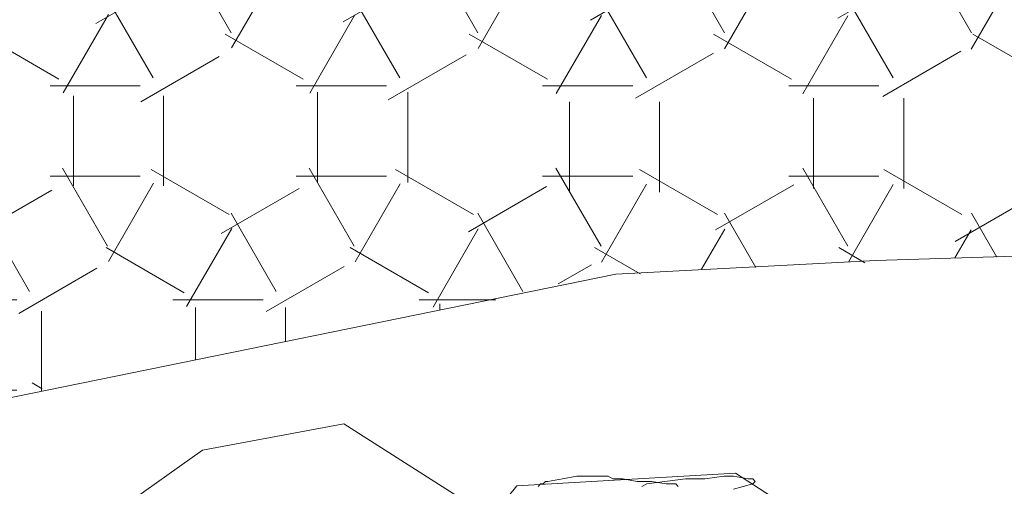
# Model space of a CAD drawing. Units: inches. Extents: x 1994 to 3075, y 3517 to 3950.
# Tile 42 of 58: x 1994.63804 to 1994.65094, y 3553.74931 to 3553.75542. Entities that reach past the tile are written whole.
import ezdxf

# ---------------------------------------------------------------- set-up
doc = ezdxf.new("R2010")
doc.units = ezdxf.units.IN
doc.layers.add('A-FURN-REFR', color=8, linetype='Continuous', lineweight=13)
doc.layers.add('A-FURN-REFR-PATT', color=8, linetype='Continuous', lineweight=13)

msp = doc.modelspace()

# ---------------------------------------------------------------- hatches: boundary and pattern name
at = {"layer": 'A-FURN-REFR-PATT'}
h = msp.add_hatch(dxfattribs=at)
h.set_pattern_fill('ESA_QT1', color=256, scale=0.001181, style=0, pattern_type=2)
h.set_pattern_definition([(0, (2000.7131367, 3549.95567), (0.0016133858, 0.0027944882), [0.0011811024, -0.0020457874]), (0, (2000.7131367, 3549.956851), (0.0016133858, 0.0027944882), [0.0011811024, -0.0020457874]), (60, (2000.7147507, 3549.9540566), (-0.0016134048, 0.0027944772), [0.0011811024, -0.0020457874]), (60, (2000.7137272, 3549.9546472), (-0.0016134048, 0.0027944772), [0.0011811024, -0.0020457874]), (120, (2000.7159311, 3549.9540566), (-0.0032267907, -1.1e-08), [0.0011811024, -0.0020457874]), (120, (2000.716954, 3549.9546472), (-0.0032267907, -1.1e-08), [0.0011811024, -0.0020457874]), (90, (2000.7131367, 3549.95567), (-0.00161338583, 0.0027944882), [0.0011811024, -0.0044079921]), (90, (2000.7143178, 3549.95567), (-0.00161338583, 0.0027944882), [0.0011811024, -0.0044079921]), (30, (2000.7159311, 3549.9540566), (0.00161340485, 0.0027944772), [0.0011811024, -0.0044079921]), (150, (2000.71475, 3549.9540566), (-0.00322679068, 1.1e-08), [0.0011811024, -0.0044079921]), (30, (2000.7153406, 3549.9550795), (0.00161340485, 0.0027944772), [0.0011811024, -0.0044079921]), (150, (2000.7153406, 3549.9550795), (-0.00322679068, 1.1e-08), [0.0011811024, -0.0044079921])])
edge = h.paths.add_edge_path()
edge.add_ellipse((1994.640876, 3553.752584), major_axis=(0, 0.019971), ratio=0.910403, start_angle=279.2385, end_angle=295.7126)
edge.add_ellipse((1994.661382, 3553.784799), major_axis=(0, 0.024564), ratio=0.910403, start_angle=170.9484, end_angle=180.8636)
edge.add_line((1994.661753, 3553.760238), (1994.660448, 3553.761168))
edge.add_line((1994.660448, 3553.761168), (1994.657839, 3553.762473))
edge.add_line((1994.657839, 3553.762473), (1994.656621, 3553.763504))
edge.add_line((1994.656621, 3553.763504), (1994.655861, 3553.763272))
edge.add_line((1994.655861, 3553.763272), (1994.655293, 3553.763476))
edge.add_line((1994.655293, 3553.763476), (1994.655493, 3553.762522))
edge.add_line((1994.655493, 3553.762522), (1994.655292, 3553.760584))
edge.add_line((1994.655292, 3553.760584), (1994.655292, 3553.760424))
edge.add_line((1994.655292, 3553.760424), (1994.655994, 3553.759788))
edge.add_line((1994.655994, 3553.759788), (1994.656079, 3553.758256))
edge.add_line((1994.656079, 3553.758256), (1994.654831, 3553.75802))
edge.add_line((1994.654831, 3553.75802), (1994.653607, 3553.75863))
edge.add_line((1994.653607, 3553.75863), (1994.651194, 3553.757931))
edge.add_line((1994.651194, 3553.757931), (1994.647697, 3553.757851))
edge.add_line((1994.647697, 3553.757851), (1994.645839, 3553.758008))
edge.add_line((1994.645839, 3553.758008), (1994.644836, 3553.757661))
edge.add_line((1994.644836, 3553.757661), (1994.64177, 3553.757379))
edge.add_line((1994.64177, 3553.757379), (1994.63952, 3553.757537))
edge.add_line((1994.63952, 3553.757537), (1994.636664, 3553.757269))
edge.add_line((1994.636664, 3553.757269), (1994.635142, 3553.757511))
edge.add_line((1994.635142, 3553.757511), (1994.634583, 3553.7569))
edge.add_line((1994.634583, 3553.7569), (1994.633061, 3553.756568))
edge.add_line((1994.633061, 3553.756568), (1994.631936, 3553.756647))
edge.add_line((1994.631936, 3553.756647), (1994.631946, 3553.757723))
edge.add_line((1994.631946, 3553.757723), (1994.632293, 3553.759053))
edge.add_line((1994.632293, 3553.759053), (1994.631942, 3553.760336))
edge.add_line((1994.631942, 3553.760336), (1994.631857, 3553.761868))
edge.add_line((1994.631857, 3553.761868), (1994.63213, 3553.76327))
edge.add_line((1994.63213, 3553.76327), (1994.632168, 3553.765117))
edge.add_line((1994.632168, 3553.765117), (1994.631874, 3553.766635))
edge.add_line((1994.631874, 3553.766635), (1994.632212, 3553.768118))
edge.add_line((1994.632212, 3553.768118), (1994.631521, 3553.769225))
edge.add_line((1994.631521, 3553.769225), (1994.631256, 3553.770206))
edge.add_line((1994.631256, 3553.770206), (1994.631719, 3553.770698))
edge.add_line((1994.631719, 3553.770698), (1994.632688, 3553.770917))
edge.add_line((1994.632688, 3553.770917), (1994.633747, 3553.770757))
edge.add_line((1994.633747, 3553.770757), (1994.63499, 3553.77107))
edge.add_line((1994.63499, 3553.77107), (1994.637864, 3553.771031))
edge.add_line((1994.637864, 3553.771031), (1994.638857, 3553.770678))
edge.add_line((1994.638857, 3553.770678), (1994.641165, 3553.770867))
edge.add_line((1994.641165, 3553.770867), (1994.645224, 3553.770907))
edge.add_line((1994.645224, 3553.770907), (1994.645865, 3553.770719))
edge.add_line((1994.645865, 3553.770719), (1994.647785, 3553.771462))
edge.add_line((1994.647785, 3553.771462), (1994.650215, 3553.771855))
edge.add_line((1994.650215, 3553.771855), (1994.65289, 3553.771785))
edge.add_line((1994.65289, 3553.771785), (1994.653416, 3553.772222))
edge.add_line((1994.653416, 3553.772222), (1994.654716, 3553.77277))
edge.add_line((1994.654716, 3553.77277), (1994.655776, 3553.77261))
edge.add_line((1994.655776, 3553.77261), (1994.655708, 3553.771299))
edge.add_line((1994.655708, 3553.771299), (1994.655135, 3553.770261))
edge.add_line((1994.655135, 3553.770261), (1994.655243, 3553.769577))
edge.add_line((1994.655243, 3553.769577), (1994.655057, 3553.767873))
edge.add_line((1994.655057, 3553.767873), (1994.655113, 3553.767736))
edge.add_line((1994.655113, 3553.767736), (1994.655702, 3553.76907))
edge.add_line((1994.655702, 3553.76907), (1994.656565, 3553.770145))
edge.add_line((1994.656565, 3553.770145), (1994.657423, 3553.771734))
edge.add_line((1994.657423, 3553.771734), (1994.657844, 3553.773215))
edge.add_line((1994.657844, 3553.773215), (1994.658028, 3553.77343))
edge.add_line((1994.658028, 3553.77343), (1994.632244, 3553.77343))
edge.add_ellipse((1994.632244, 3553.771319), major_axis=(0, 0.002111), ratio=0.910403, start_angle=0, end_angle=90)
edge.add_line((1994.630322, 3553.771319), (1994.630322, 3553.749441))
edge.add_line((1994.630322, 3553.749441), (1994.637709, 3553.750433))
edge.add_line((1994.637709, 3553.750433), (1994.645849, 3553.752088))
edge.add_line((1994.645849, 3553.752088), (1994.649254, 3553.75227))
edge.add_line((1994.649254, 3553.75227), (1994.654398, 3553.752423))
edge.add_line((1994.654398, 3553.752423), (1994.656593, 3553.752621))
edge.add_ellipse((1994.639937, 3553.760628), major_axis=(0, 0.019971), ratio=0.910403, start_angle=244.323, end_angle=253.1594)
edge.add_ellipse((1994.674344, 3553.771437), major_axis=(0, 0.024564), ratio=0.910403, start_angle=133.6721, end_angle=139.6806)
edge.add_line((1994.659095, 3553.753469), (1994.658861, 3553.755509))
edge = h.paths.add_edge_path()
edge.add_ellipse((1994.680284, 3553.771319), major_axis=(0, 0.002111), ratio=0.910403, start_angle=270, end_angle=360)
edge.add_line((1994.680284, 3553.77343), (1994.665356, 3553.77343))
edge.add_line((1994.665356, 3553.77343), (1994.665734, 3553.77298))
edge.add_line((1994.665734, 3553.77298), (1994.66783, 3553.771902))
edge.add_line((1994.66783, 3553.771902), (1994.671387, 3553.769751))
edge.add_line((1994.671387, 3553.769751), (1994.671861, 3553.769242))
edge.add_line((1994.671861, 3553.769242), (1994.673866, 3553.768856))
edge.add_line((1994.673866, 3553.768856), (1994.676159, 3553.76789))
edge.add_line((1994.676159, 3553.76789), (1994.67846, 3553.766389))
edge.add_line((1994.67846, 3553.766389), (1994.679113, 3553.766487))
edge.add_line((1994.679113, 3553.766487), (1994.680491, 3553.766264))
edge.add_line((1994.680491, 3553.766264), (1994.681343, 3553.765554))
edge.add_line((1994.681343, 3553.765554), (1994.680699, 3553.764448))
edge.add_line((1994.680699, 3553.764448), (1994.679737, 3553.763852))
edge.add_line((1994.679737, 3553.763852), (1994.679525, 3553.763197))
edge.add_line((1994.679525, 3553.763197), (1994.678603, 3553.761813))
edge.add_line((1994.678603, 3553.761813), (1994.678548, 3553.76116))
edge.add_line((1994.678548, 3553.76116), (1994.678066, 3553.759541))
edge.add_line((1994.678066, 3553.759541), (1994.676936, 3553.75803))
edge.add_line((1994.676936, 3553.75803), (1994.676848, 3553.757857))
edge.add_line((1994.676848, 3553.757857), (1994.676595, 3553.756914))
edge.add_line((1994.676595, 3553.756914), (1994.675477, 3553.755213))
edge.add_line((1994.675477, 3553.755213), (1994.675812, 3553.754261))
edge.add_line((1994.675812, 3553.754261), (1994.675202, 3553.75288))
edge.add_line((1994.675202, 3553.75288), (1994.674009, 3553.753346))
edge.add_line((1994.674009, 3553.753346), (1994.673214, 3553.754537))
edge.add_line((1994.673214, 3553.754537), (1994.670799, 3553.755226))
edge.add_line((1994.670799, 3553.755226), (1994.66897, 3553.756302))
edge.add_ellipse((1994.691382, 3553.757287), major_axis=(0, 0.024638), ratio=0.910403, start_angle=92.5166, end_angle=102.9728)
edge.add_line((1994.66943, 3553.75223), (1994.673814, 3553.75171))
edge.add_line((1994.673814, 3553.75171), (1994.677653, 3553.751587))
edge.add_line((1994.677653, 3553.751587), (1994.682205, 3553.751587))
edge.add_line((1994.682205, 3553.751587), (1994.682205, 3553.755102))
edge.add_line((1994.682205, 3553.755102), (1994.682205, 3553.771319))

# ---------------------------------------------------------------- linework, layer by layer
at = {"layer": 'A-FURN-REFR'}
for p, q in [((1994.649254, 3553.75227), (1994.654398, 3553.752423)), ((1994.645849, 3553.752088), (1994.649254, 3553.75227)), ((1994.637709, 3553.750433), (1994.645849, 3553.752088)), ((1994.640431, 3553.749786), (1994.642283, 3553.750132)), ((1994.642283, 3553.750132), (1994.644212, 3553.748903)), ((1994.638001, 3553.748064), (1994.640431, 3553.749786)), ((1994.644551, 3553.749317), (1994.647417, 3553.749486)), ((1994.645336, 3553.749447), (1994.645147, 3553.749412)), ((1994.645747, 3553.749447), (1994.645336, 3553.749447)), ((1994.64581, 3553.749412), (1994.645747, 3553.749447)), ((1994.647012, 3553.749412), (1994.647265, 3553.749447)), ((1994.647265, 3553.749447), (1994.647391, 3553.749447)), ((1994.647391, 3553.749447), (1994.647581, 3553.749412)), ((1994.647417, 3553.749486), (1994.649645, 3553.748037)), ((1994.644212, 3553.748903), (1994.644551, 3553.749317)), ((1994.644862, 3553.749343), (1994.644831, 3553.749308)), ((1994.644894, 3553.749343), (1994.644862, 3553.749343)), ((1994.644925, 3553.749377), (1994.644894, 3553.749343)), ((1994.644957, 3553.749377), (1994.644925, 3553.749377)), ((1994.645147, 3553.749412), (1994.644957, 3553.749377)), ((1994.645937, 3553.749412), (1994.64581, 3553.749412)), ((1994.646127, 3553.749377), (1994.645937, 3553.749412)), ((1994.646316, 3553.749377), (1994.646127, 3553.749377)), ((1994.64619, 3553.749308), (1994.646253, 3553.749343)), ((1994.646253, 3553.749343), (1994.646759, 3553.749412)), ((1994.646506, 3553.749343), (1994.646316, 3553.749377)), ((1994.646632, 3553.749343), (1994.646506, 3553.749343)), ((1994.646664, 3553.749308), (1994.646632, 3553.749343)), ((1994.646759, 3553.749412), (1994.647012, 3553.749412)), ((1994.647644, 3553.749343), (1994.647391, 3553.749273)), ((1994.647581, 3553.749412), (1994.647644, 3553.749412)), ((1994.647644, 3553.749412), (1994.647675, 3553.749377)), ((1994.647675, 3553.749377), (1994.647644, 3553.749343))]:
    msp.add_line(p, q, dxfattribs=at)

doc.saveas('drawing.dxf')
